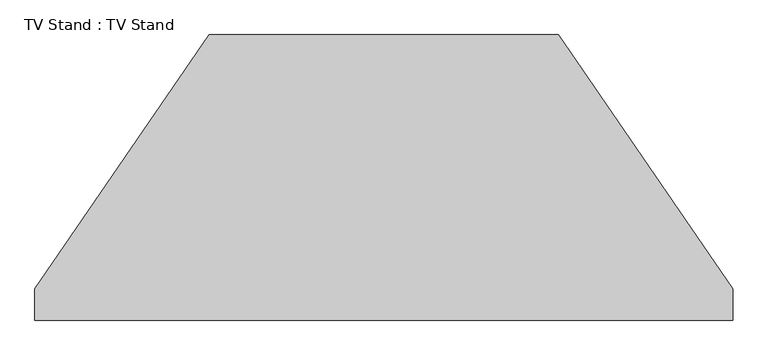
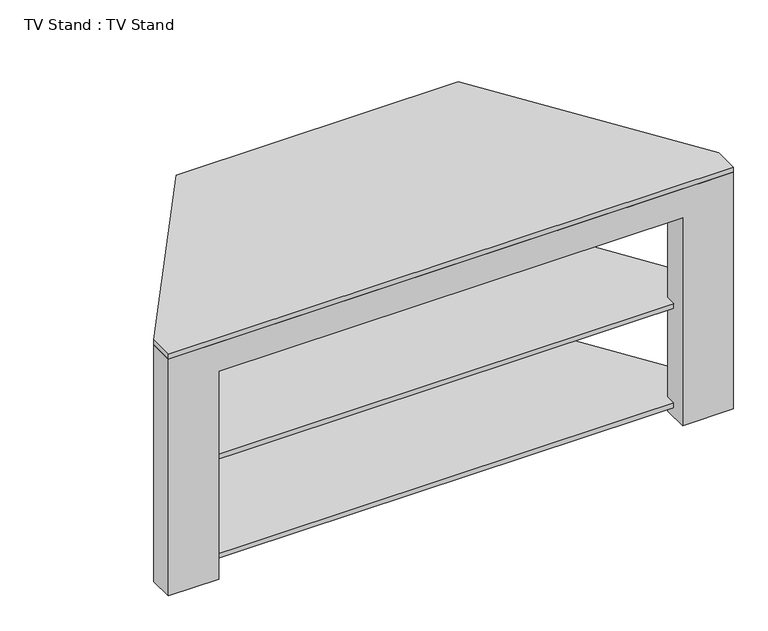
"""IFC4 building model written with IfcOpenShell, lengths in millimetres: furniture geometry, TV Stand : TV Stand."""

from ifc_helpers import new_model, si_unit, point, frame, frame_2d, origin, place, context, project, spatial, polyline, circle_curve, trimmed, segment, composite_curve, outline, extrude, faceted_brep, source, transform, mapped, element, save


def tv_stand_tv_stand_6ac32a77(model_context):
    return source(origin(), model_context, "Body", "SolidModel", [
        extrude(outline(polyline([(0.0, 304.5880021), (495.3, 304.5880021), (495.3, -54.2119979), (0.0, -54.2119979), (0.0, 304.5880021)]), holes=[composite_curve([segment(polyline([(242.65, 145.1700818), (242.65, 105.2059224)]), True, "CONTINUOUS"), segment(trimmed(circle_curve(frame_2d((255.15, 105.2059224)), 12.5), [point((242.65, 105.2059224))], [point((267.65, 105.2059224))], True, "CARTESIAN"), True, "CONTINUOUS"), segment(polyline([(267.65, 105.2059224), (267.65, 145.1700818)]), True, "CONTINUOUS"), segment(trimmed(circle_curve(frame_2d((255.15, 145.1700818)), 12.5), [point((267.65, 145.1700818))], [point((242.65, 145.1700818))], True, "CARTESIAN"), True, "CONTINUOUS")], self_intersect=False), composite_curve([segment(polyline([(35.0, 145.1880021), (35.0, 105.2059224)]), True, "CONTINUOUS"), segment(trimmed(circle_curve(frame_2d((47.5, 105.2059224)), 12.5), [point((35.0, 105.2059224))], [point((60.0, 105.2059224))], True, "CARTESIAN"), True, "CONTINUOUS"), segment(polyline([(60.0, 105.2059224), (60.0, 145.1880021)]), True, "CONTINUOUS"), segment(trimmed(circle_curve(frame_2d((47.5, 145.1880021)), 12.5), [point((60.0, 145.1880021))], [point((35.0, 145.1880021))], True, "CARTESIAN"), True, "CONTINUOUS")], self_intersect=False)]), frame((0.0, -30.0, 0.0), z_axis=(0.0, 1.0, 0.0), x_axis=(0.0, 0.0, 1.0)), (0.0, 0.0, 1.0), 10.0),
        faceted_brep([(-433.6119979, -457.2, 0.0), (-333.6119979, -457.2, 0.0), (-333.6119979, -457.2, 435.3), (583.9880021, -457.2, 435.3), (583.9880021, -457.2, 0.0), (683.9880021, -457.2, 0.0), (683.9880021, -457.2, 495.3), (-433.6119979, -457.2, 495.3), (-433.6119979, -407.2, 0.0), (-433.6119979, -407.2, 495.3), (683.9880021, -407.2, 495.3), (683.9880021, -407.2, 0.0), (583.9880021, -407.2, 0.0), (583.9880021, -407.2, 20.0), (633.9880021, -407.2, 20.0), (633.9880021, -407.2, 30.0), (583.9880021, -407.2, 30.0), (583.9880021, -407.2, 227.65), (633.9880021, -407.2, 227.65), (633.9880021, -407.2, 237.65), (583.9880021, -407.2, 237.65), (583.9880021, -407.2, 435.3), (-333.6119979, -407.2, 435.3), (-333.6119979, -407.2, 237.65), (-383.6119979, -407.2, 237.65), (-383.6119979, -407.2, 227.65), (-333.6119979, -407.2, 227.65), (-333.6119979, -407.2, 30.0), (-383.6119979, -407.2, 30.0), (-383.6119979, -407.2, 20.0), (-333.6119979, -407.2, 20.0), (-333.6119979, -407.2, 0.0), (-333.6119979, -427.2, 20.0), (-333.6119979, -427.2, 30.0), (-333.6119979, -427.2, 227.65), (-333.6119979, -427.2, 237.65), (583.9880021, -427.2, 237.65), (583.9880021, -427.2, 227.65), (583.9880021, -427.2, 30.0), (583.9880021, -427.2, 20.0), (633.9880021, -427.2, 237.65), (-383.6119979, -427.2, 237.65), (-383.6119979, -427.2, 227.65), (633.9880021, -427.2, 227.65), (633.9880021, -427.2, 30.0), (-383.6119979, -427.2, 30.0), (-383.6119979, -427.2, 20.0), (633.9880021, -427.2, 20.0)], [[[0, 1, 2, 3, 4, 5, 6, 7]], [[8, 9, 10, 11, 12, 13, 14, 15, 16, 17, 18, 19, 20, 21, 22, 23, 24, 25, 26, 27, 28, 29, 30, 31]], [[1, 0, 8, 31]], [[2, 1, 31, 30, 32, 33, 27, 26, 34, 35, 23, 22]], [[3, 2, 22, 21]], [[4, 3, 21, 20, 36, 37, 17, 16, 38, 39, 13, 12]], [[5, 4, 12, 11]], [[6, 5, 11, 10]], [[7, 6, 10, 9]], [[0, 7, 9, 8]], [[19, 40, 36, 20]], [[35, 41, 24, 23]], [[25, 42, 34, 26]], [[37, 43, 18, 17]], [[41, 42, 25, 24]], [[42, 41, 35, 34]], [[40, 43, 37, 36]], [[43, 40, 19, 18]], [[15, 44, 38, 16]], [[33, 45, 28, 27]], [[29, 46, 32, 30]], [[39, 47, 14, 13]], [[45, 46, 29, 28]], [[46, 45, 33, 32]], [[44, 47, 39, 38]], [[47, 44, 15, 14]]]),
        extrude(outline(polyline([(-50.0, 495.3), (0.0, 495.3), (0.0, 0.0), (-50.0, 0.0), (-50.0, 20.0), (-30.0, 20.0), (-30.0, 30.0), (-50.0, 30.0), (-50.0, 227.65), (-30.0, 227.65), (-30.0, 237.65), (-50.0, 237.65), (-50.0, 495.3)])), frame((-154.2119979, 0.0, 0.0), z_axis=(1.0, 0.0, 0.0), x_axis=(0.0, 1.0, 0.0)), (0.0, 0.0, 1.0), 100.0),
        extrude(outline(polyline([(-50.0, 495.3), (0.0, 495.3), (0.0, 0.0), (-50.0, 0.0), (-50.0, 20.0), (-30.0, 20.0), (-30.0, 30.0), (-50.0, 30.0), (-50.0, 227.65), (-30.0, 227.65), (-30.0, 237.65), (-50.0, 237.65), (-50.0, 495.3)])), frame((304.5880021, 0.0, 0.0), z_axis=(1.0, 0.0, 0.0), x_axis=(0.0, 1.0, 0.0)), (0.0, 0.0, 1.0), 100.0),
        extrude(outline(polyline([(404.5880021, 0.0), (683.9880021, -407.2), (683.9880021, -457.2), (-433.6119979, -457.2), (-433.6119979, -407.2), (-154.2119979, 0.0), (404.5880021, 0.0)])), frame((0.0, 0.0, 495.3), z_axis=(0.0, 0.0, 1.0), x_axis=(1.0, 0.0, 0.0)), (0.0, 0.0, 1.0), 10.0),
        extrude(outline(polyline([(425.1724814, -30.0), (633.9880021, -334.3295634), (633.9880021, -427.2), (-383.6119979, -427.2), (-383.6119979, -334.3295634), (-174.7964773, -30.0), (425.1724814, -30.0)])), frame((0.0, 0.0, 227.65), z_axis=(0.0, 0.0, 1.0), x_axis=(1.0, 0.0, 0.0)), (0.0, 0.0, 1.0), 10.0),
        extrude(outline(polyline([(425.1724814, -30.0), (633.9880021, -334.3295634), (633.9880021, -427.2), (-383.6119979, -427.2), (-383.6119979, -334.3295634), (-174.7964773, -30.0), (425.1724814, -30.0)])), frame((0.0, 0.0, 20.0), z_axis=(0.0, 0.0, 1.0), x_axis=(1.0, 0.0, 0.0)), (0.0, 0.0, 1.0), 10.0),
    ])


if __name__ == "__main__":
    model = new_model("IFC4")
    model_context = context("Model", 3, world=origin())
    ifc_project = project(units=[si_unit("LENGTHUNIT", "METRE", prefix="MILLI")], contexts=[model_context])
    site = spatial("IfcSite", under=ifc_project)
    building = spatial("IfcBuilding", under=site)
    placement = place(None, origin())
    tv_stand_tv_stand_shape = tv_stand_tv_stand_6ac32a77(model_context)
    element("IfcFurniture", 1, ObjectType="TV Stand : TV Stand", at=placement, inside=building, context=model_context, shape_type="MappedRepresentation", body=[
        mapped(tv_stand_tv_stand_shape, transform((0.0, 0.0, 0.0), x_axis=(1.0, 0.0, 0.0), y_axis=(0.0, 1.0, 0.0), z_axis=(0.0, 0.0, 1.0))),
    ])
    save(model, "model.ifc")

# Revit data of these elements
# Type "TV Stand : TV Stand"
#   Depth = 1' - 6"
#   Width = 3' - 8"
#   Height = 1' - 7 1/2"
#   Finish = Melamine - Gray
#   Default Elevation = 0
# Element 1 (IfcFurniture, "TV Stand : TV Stand")
#   Materials on its faces: "Melamine - Gray", "Glass - Shelves"
# Materials
#   "Melamine - Gray": class "Wood", colour RGB 49 49 49, transparency 0
#   "Glass - Shelves": class "Glass", colour RGB 167 167 167, transparency 0.9
